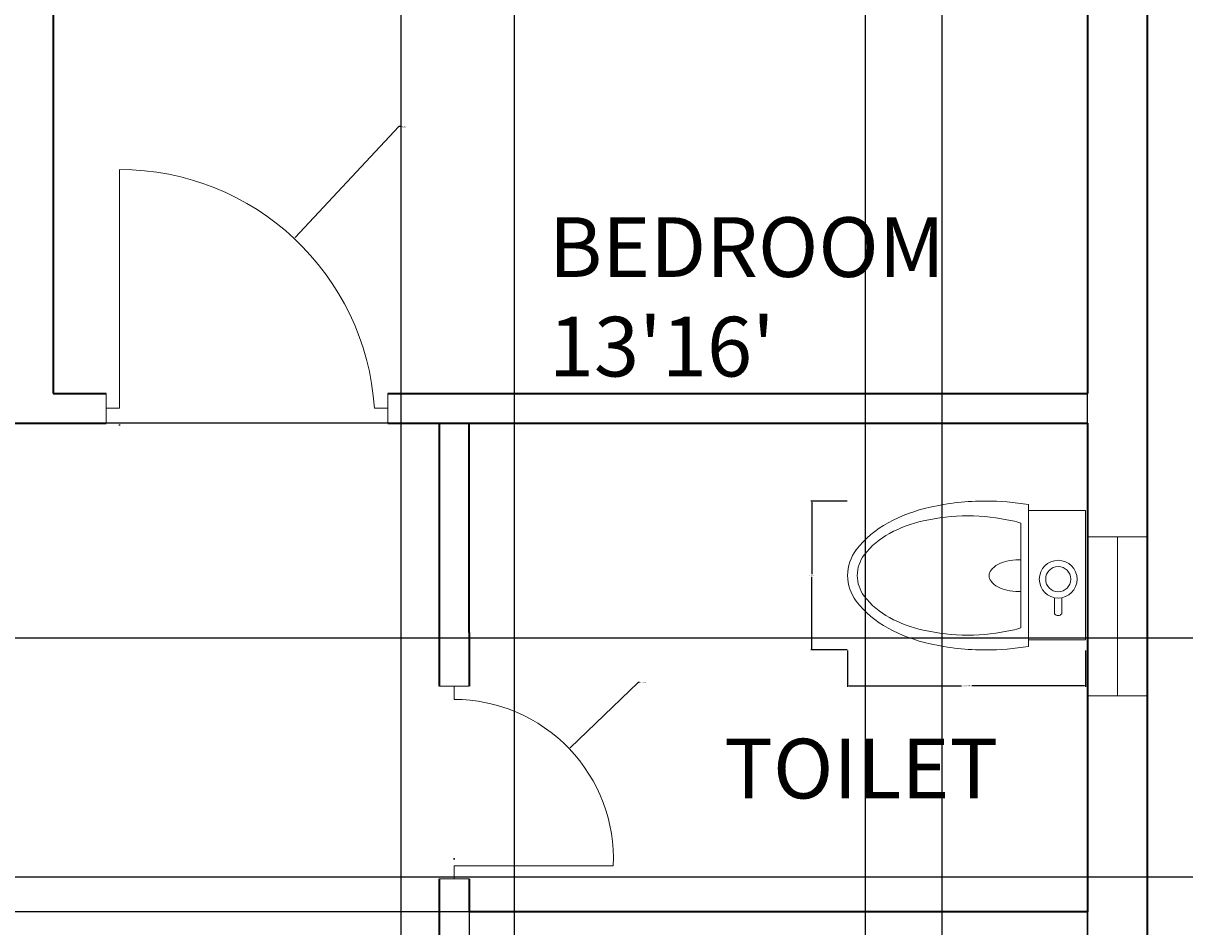
# Model space of a CAD drawing. Units: inches. Extents: x 1770 to 2988, y 1161 to 3221.
# Tile 22 of 44: x 2456 to 2631, y 2095 to 2231. Entities that reach past the tile are written whole.
import ezdxf

# ---------------------------------------------------------------- set-up
doc = ezdxf.new("R2010")
doc.units = ezdxf.units.IN
for name, color, linetype, lineweight in [('A-ANNO-DIMS', 2, 'Continuous', 18), ('A-AREA-IDEN', 7, 'Continuous', 18), ('A-DOOR', 4, 'Continuous', 18), ('A-FLOR-FIXT', 9, 'Continuous', 18), ('A-GLAZ', 4, 'Continuous', 18), ('A-WALL', 7, 'Continuous', 35)]:
    doc.layers.add(name, color=color, linetype=linetype, lineweight=lineweight)
doc.styles.get("Standard").update_dxf_attribs({"font": 'arial.ttf'})
doc.dimstyles.get("Standard").update_dxf_attribs({"dimtxt": 0.18, "dimasz": 0.18, "dimexe": 0.18, "dimexo": 0.0625, "dimgap": 0.09, "dimtad": 0, "dimtih": 1, "dimtoh": 1, "dimdec": 4, "dimzin": 0, "dimdsep": 46, "dimtxsty": 'Standard', "dimcen": 0.09, "dimadec": 0, "dimazin": 0, "dimtfac": 1, "dimtdec": 4, "dimtofl": 0, "dimtmove": 0, "dimatfit": 3, "dimfxl": 1, "dimtolj": 1, "dimtzin": 0, "dimarcsym": 0})

# ---------------------------------------------------------------- blocks, each defined once
blk = doc.blocks.new('A$C7FD35E1A')
for p, q in [((0.0233, 0.5799), (0.0233, 0.4408)), ((0.0233, 0.5799), (0.338, 0.5799)), ((0.338, 0.5799), (0.338, 0.4408)), ((0.2357, 0.5217), (0.2745, 0.5217)), ((0.2356, 0.5044), (0.275, 0.5044)), ((0.3542, 0.4408), (0.0087, 0.4408)), ((0.3093, 0.4224), (0.0536, 0.4224))]:
    blk.add_line(p, q)
for radius in [0.046, 0.0305]:
    blk.add_circle((0.1904, 0.5132), radius)
for centre, radius, start, end in [((0.2685, 0.5129), 0.0107, 307.488, 55.394), ((0.6238, 0.337), 0.6238, 170.4184, 180), ((-0.261, 0.337), 0.6238, 0, 9.5816), ((0.5354, 0.2931), 0.4991, 167.4267, 180), ((0.3603, 0.3321), 0.3197, 163.5954, 167.4267), ((0.277, 0.4171), 0.1337, 177.7133, 180), ((0.277, 0.4171), 0.1337, 180, 192.5399), ((0.0869, 0.4171), 0.1337, 347.4601, 0), ((0.0869, 0.4171), 0.1337, 360, 2.2867), ((0.0026, 0.3321), 0.3197, 12.5733, 16.4046), ((-0.1725, 0.2931), 0.4991, 0, 12.5733), ((0.23, 0.4066), 0.0855, 192.5399, 208.2349), ((0.1339, 0.4066), 0.0855, 331.7651, 347.4601), ((0.2004, 0.3907), 0.052, 208.2349, 232.3543), ((0.182, 0.3668), 0.0218, 232.3543, 270), ((0.182, 0.3668), 0.0218, 270, 307.6457), ((0.1635, 0.3907), 0.052, 307.6457, 331.7651), ((0.6238, 0.337), 0.6238, 180, 192.5733), ((-0.261, 0.337), 0.6238, 347.4267, 0), ((0.5354, 0.2931), 0.4991, 180, 192.5733), ((-0.1725, 0.2931), 0.4991, 347.4267, 0), ((0.405, 0.2881), 0.3996, 192.5733, 208.3008), ((-0.0421, 0.2881), 0.3996, 331.6992, 347.4267), ((0.3603, 0.254), 0.3197, 192.5733, 208.3008), ((0.0026, 0.254), 0.3197, 331.6992, 347.4267), ((0.2672, 0.214), 0.2432, 208.3008, 232.4306), ((0.2501, 0.1947), 0.1945, 208.3008, 232.4306), ((0.1128, 0.1947), 0.1945, 307.5694, 331.6992), ((0.0957, 0.214), 0.2432, 307.5694, 331.6992), ((0.1814, 0.1055), 0.082, 232.4306, 270), ((0.1814, 0.1055), 0.082, 270, 307.5694), ((0.1814, 0.1024), 0.1024, 232.4306, 270), ((0.1814, 0.1024), 0.1024, 270, 307.5694)]:
    blk.add_arc(centre, radius, start, end)
blk = doc.blocks.new('WIN-24-EXT')
for p, q in [((0, 9), (0, 0)), ((24, 4.5), (24, 9)), ((24, 9), (24, 0)), ((0, 0), (0, 4.5)), ((0, 4.5), (24, 4.5))]:
    blk.add_line(p, q)
blk = doc.blocks.new('*D40')
at = {"layer": 'A-ANNO-DIMS', "color": 0, "lineweight": -2, "transparency": 16777216}
for p, q in [((2580.5, 2136.95), (2580.5, 2131.45)), ((2616.39, 2136.95), (2616.39, 2131.45)), ((2580.68, 2131.63), (2597.67, 2131.63)), ((2616.21, 2131.63), (2599.22, 2131.63))]:
    blk.add_line(p, q, dxfattribs=at)
at = {"layer": 'A-ANNO-DIMS', "color": 0, "transparency": 16777216}
for points in [[(2580.68, 2131.66), (2580.68, 2131.6), (2580.5, 2131.63)], [(2616.21, 2131.66), (2616.21, 2131.6), (2616.39, 2131.63)]]:
    blk.add_solid(points, dxfattribs=at)
at = {"layer": 'Defpoints', "color": 0, "transparency": 16777216}
for p in [(2580.5, 2137.02), (2616.39, 2137.02), (2616.39, 2131.63)]:
    blk.add_point(p, dxfattribs=at)
at = {"layer": 'A-ANNO-DIMS', "color": 0, "transparency": 16777216, "insert": (2598.45, 2131.63), "char_height": 0.18, "attachment_point": 5}
blk.add_mtext('\\A1;WC 36 TYP.', dxfattribs=at)
blk = doc.blocks.new('*D41')
at = {"layer": 'A-ANNO-DIMS', "color": 0, "lineweight": -2, "transparency": 16777216}
for p, q in [((2580.44, 2159.47), (2574.94, 2159.47)), ((2575.12, 2159.29), (2575.12, 2148.43)), ((2575.12, 2137.2), (2575.12, 2148.07)), ((2580.44, 2137.02), (2574.94, 2137.02))]:
    blk.add_line(p, q, dxfattribs=at)
at = {"layer": 'A-ANNO-DIMS', "color": 0, "transparency": 16777216}
for points in [[(2575.09, 2159.29), (2575.15, 2159.29), (2575.12, 2159.47)], [(2575.09, 2137.2), (2575.15, 2137.2), (2575.12, 2137.02)]]:
    blk.add_solid(points, dxfattribs=at)
at = {"layer": 'Defpoints', "color": 0, "transparency": 16777216}
for p in [(2580.5, 2159.47), (2575.12, 2137.02), (2580.5, 2137.02)]:
    blk.add_point(p, dxfattribs=at)
at = {"layer": 'A-ANNO-DIMS', "color": 0, "transparency": 16777216, "insert": (2575.12, 2148.25), "char_height": 0.18, "attachment_point": 5}
blk.add_mtext('\\A1;22 TYP.', dxfattribs=at)
blk = doc.blocks.new('*D61')
at = {"layer": 'A-ANNO-DIMS', "color": 0, "lineweight": -2, "transparency": 16777216}
for p, q in [((2625.76, 2376.7), (2866.87, 2376.7)), ((2866.69, 2376.52), (2866.69, 1993.63)), ((2866.69, 1610.38), (2866.69, 1993.27)), ((2625.76, 1610.2), (2866.87, 1610.2))]:
    blk.add_line(p, q, dxfattribs=at)
at = {"layer": 'A-ANNO-DIMS', "color": 0, "transparency": 16777216}
for points in [[(2866.66, 2376.52), (2866.72, 2376.52), (2866.69, 2376.7)], [(2866.66, 1610.38), (2866.72, 1610.38), (2866.69, 1610.2)]]:
    blk.add_solid(points, dxfattribs=at)
at = {"layer": 'Defpoints', "color": 0, "transparency": 16777216}
for p in [(2625.7, 2376.7), (2866.69, 2376.7), (2625.7, 1610.2)]:
    blk.add_point(p, dxfattribs=at)
at = {"layer": 'A-ANNO-DIMS', "color": 0, "transparency": 16777216, "insert": (2866.69, 1993.45), "char_height": 0.18, "attachment_point": 5}
blk.add_mtext('\\A1;766.5', dxfattribs=at)
blk = doc.blocks.new('*D74')
at = {"layer": 'A-ANNO-DIMS', "color": 0, "lineweight": -2, "transparency": 16777216}
for p, q in [((2523.42, 2097.48), (2523.42, 1165.57)), ((2616.7, 2097.48), (2616.7, 1165.57)), ((2523.6, 1165.75), (2569.66, 1165.75)), ((2616.52, 1165.75), (2570.45, 1165.75))]:
    blk.add_line(p, q, dxfattribs=at)
at = {"layer": 'A-ANNO-DIMS', "color": 0, "transparency": 16777216}
for points in [[(2523.6, 1165.78), (2523.6, 1165.72), (2523.42, 1165.75)], [(2616.52, 1165.78), (2616.52, 1165.72), (2616.7, 1165.75)]]:
    blk.add_solid(points, dxfattribs=at)
at = {"layer": 'Defpoints', "color": 0, "transparency": 16777216}
for p in [(2523.42, 2097.54), (2616.7, 2097.54), (2616.7, 1165.75)]:
    blk.add_point(p, dxfattribs=at)
at = {"layer": 'A-ANNO-DIMS', "color": 0, "transparency": 16777216, "insert": (2570.06, 1165.75), "char_height": 0.18, "attachment_point": 5}
blk.add_mtext('\\A1;93.28', dxfattribs=at)
blk = doc.blocks.new('*D75')
at = {"layer": 'A-ANNO-DIMS', "color": 0, "lineweight": -2, "transparency": 16777216}
for p, q in [((2523.36, 2171.2), (1907.1, 2171.2)), ((1907.28, 2171.02), (1907.28, 2134.56)), ((1907.28, 2097.72), (1907.28, 2134.19)), ((2523.36, 2097.54), (1907.1, 2097.54))]:
    blk.add_line(p, q, dxfattribs=at)
at = {"layer": 'A-ANNO-DIMS', "color": 0, "transparency": 16777216}
for points in [[(1907.25, 2171.02), (1907.31, 2171.02), (1907.28, 2171.2)], [(1907.25, 2097.72), (1907.31, 2097.72), (1907.28, 2097.54)]]:
    blk.add_solid(points, dxfattribs=at)
at = {"layer": 'Defpoints', "color": 0, "transparency": 16777216}
for p in [(2523.42, 2171.2), (1907.28, 2097.54), (2523.42, 2097.54)]:
    blk.add_point(p, dxfattribs=at)
at = {"layer": 'A-ANNO-DIMS', "color": 0, "transparency": 16777216, "insert": (1907.28, 2134.37), "char_height": 0.18, "attachment_point": 5}
blk.add_mtext('\\A1;73.66', dxfattribs=at)
blk = doc.blocks.new('*D82')
at = {"layer": 'A-ANNO-DIMS', "color": 0, "lineweight": -2, "transparency": 16777216}
for p, q in [((2443.39, 1610.26), (2443.39, 2570.7)), ((2443.57, 2570.52), (2486.45, 2570.52)), ((2530.12, 2570.52), (2487.24, 2570.52)), ((2530.3, 1610.26), (2530.3, 2570.7))]:
    blk.add_line(p, q, dxfattribs=at)
at = {"layer": 'A-ANNO-DIMS', "color": 0, "transparency": 16777216}
for points in [[(2443.57, 2570.55), (2443.57, 2570.49), (2443.39, 2570.52)], [(2530.12, 2570.55), (2530.12, 2570.49), (2530.3, 2570.52)]]:
    blk.add_solid(points, dxfattribs=at)
at = {"layer": 'Defpoints', "color": 0, "transparency": 16777216}
for p in [(2530.3, 2570.52), (2443.39, 1610.2), (2530.3, 1610.2)]:
    blk.add_point(p, dxfattribs=at)
at = {"layer": 'A-ANNO-DIMS', "color": 0, "transparency": 16777216, "insert": (2486.85, 2570.52), "char_height": 0.18, "attachment_point": 5}
blk.add_mtext('\\A1;86.92', dxfattribs=at)
blk = doc.blocks.new('*D84')
at = {"layer": 'A-ANNO-DIMS', "color": 0, "lineweight": -2, "transparency": 16777216}
for p, q in [((2513.2, 1835.26), (2513.2, 2570.7)), ((2513.38, 2570.52), (2564.56, 2570.52)), ((2616.52, 2570.52), (2565.33, 2570.52)), ((2616.7, 1835.26), (2616.7, 2570.7))]:
    blk.add_line(p, q, dxfattribs=at)
at = {"layer": 'A-ANNO-DIMS', "color": 0, "transparency": 16777216}
for points in [[(2513.38, 2570.55), (2513.38, 2570.49), (2513.2, 2570.52)], [(2616.52, 2570.55), (2616.52, 2570.49), (2616.7, 2570.52)]]:
    blk.add_solid(points, dxfattribs=at)
at = {"layer": 'Defpoints', "color": 0, "transparency": 16777216}
for p in [(2616.7, 2570.52), (2513.2, 1835.2), (2616.7, 1835.2)]:
    blk.add_point(p, dxfattribs=at)
at = {"layer": 'A-ANNO-DIMS', "color": 0, "transparency": 16777216, "insert": (2564.95, 2570.52), "char_height": 0.18, "attachment_point": 5}
blk.add_mtext('\\A1;103.5', dxfattribs=at)
blk = doc.blocks.new('*D86')
at = {"layer": 'A-ANNO-DIMS', "color": 0, "lineweight": -2, "transparency": 16777216}
for p, q in [((2583.2, 1775.21), (2583.2, 2570.7)), ((2583.38, 2570.52), (2599.62, 2570.52)), ((2616.52, 2570.52), (2600.27, 2570.52)), ((2616.7, 1775.26), (2616.7, 2570.7))]:
    blk.add_line(p, q, dxfattribs=at)
at = {"layer": 'A-ANNO-DIMS', "color": 0, "transparency": 16777216}
for points in [[(2583.38, 2570.55), (2583.38, 2570.49), (2583.2, 2570.52)], [(2616.52, 2570.55), (2616.52, 2570.49), (2616.7, 2570.52)]]:
    blk.add_solid(points, dxfattribs=at)
at = {"layer": 'Defpoints', "color": 0, "transparency": 16777216}
for p in [(2616.7, 2570.52), (2583.2, 1775.15), (2616.7, 1775.2)]:
    blk.add_point(p, dxfattribs=at)
at = {"layer": 'A-ANNO-DIMS', "color": 0, "transparency": 16777216, "insert": (2599.95, 2570.52), "char_height": 0.18, "attachment_point": 5}
blk.add_mtext('\\A1;33.5', dxfattribs=at)
blk = doc.blocks.new('*D87')
at = {"layer": 'A-ANNO-DIMS', "color": 0, "lineweight": -2, "transparency": 16777216}
for p, q in [((2594.75, 1861.4), (2594.75, 2570.7)), ((2594.93, 2570.52), (2605.33, 2570.52)), ((2616.52, 2570.52), (2606.12, 2570.52)), ((2616.7, 1839.76), (2616.7, 2570.7))]:
    blk.add_line(p, q, dxfattribs=at)
at = {"layer": 'A-ANNO-DIMS', "color": 0, "transparency": 16777216}
for points in [[(2594.93, 2570.55), (2594.93, 2570.49), (2594.75, 2570.52)], [(2616.52, 2570.55), (2616.52, 2570.49), (2616.7, 2570.52)]]:
    blk.add_solid(points, dxfattribs=at)
at = {"layer": 'Defpoints', "color": 0, "transparency": 16777216}
for p in [(2616.7, 2570.52), (2594.75, 1861.34), (2616.7, 1839.7)]:
    blk.add_point(p, dxfattribs=at)
at = {"layer": 'A-ANNO-DIMS', "color": 0, "transparency": 16777216, "insert": (2605.72, 2570.52), "char_height": 0.18, "attachment_point": 5}
blk.add_mtext('\\A1;21.95', dxfattribs=at)
blk = doc.blocks.new('*D89')
at = {"layer": 'A-ANNO-DIMS', "color": 0, "lineweight": -2, "transparency": 16777216}
for p, q in [((2160.76, 2138.84), (2866.87, 2138.84)), ((2866.69, 2138.66), (2866.69, 2121.02)), ((2866.69, 2103.02), (2866.69, 2120.66)), ((2160.76, 2102.84), (2866.87, 2102.84))]:
    blk.add_line(p, q, dxfattribs=at)
at = {"layer": 'A-ANNO-DIMS', "color": 0, "transparency": 16777216}
for points in [[(2866.66, 2138.66), (2866.72, 2138.66), (2866.69, 2138.84)], [(2866.66, 2103.02), (2866.72, 2103.02), (2866.69, 2102.84)]]:
    blk.add_solid(points, dxfattribs=at)
at = {"layer": 'Defpoints', "color": 0, "transparency": 16777216}
for p in [(2160.7, 2138.84), (2866.69, 2138.84), (2160.7, 2102.84)]:
    blk.add_point(p, dxfattribs=at)
at = {"layer": 'A-ANNO-DIMS', "color": 0, "transparency": 16777216, "insert": (2866.69, 2120.84), "char_height": 0.18, "attachment_point": 5}
blk.add_mtext('\\A1;36', dxfattribs=at)
blk = doc.blocks.new('*D111')
at = {"layer": 'A-ANNO-DIMS', "color": 0, "lineweight": -2, "transparency": 16777216}
for p, q in [((2512.85, 2215.91), (2497.18, 2199.18)), ((2513.03, 2215.91), (2512.85, 2215.91)), ((2470.64, 2170.94), (2470.82, 2170.94)), ((2470.73, 2170.85), (2470.73, 2171.03))]:
    blk.add_line(p, q, dxfattribs=at)
at = {"layer": 'A-ANNO-DIMS', "color": 0, "transparency": 16777216}
blk.add_solid([(2497.16, 2199.2), (2497.2, 2199.16), (2497.06, 2199.05)], dxfattribs=at)
at = {"layer": 'Defpoints', "color": 0, "transparency": 16777216}
for p in [(2497.06, 2199.05), (2470.73, 2170.94)]:
    blk.add_point(p, dxfattribs=at)
at = {"layer": 'A-ANNO-DIMS', "color": 0, "transparency": 16777216, "insert": (2513.5, 2215.91), "char_height": 0.18, "attachment_point": 5}
blk.add_mtext('\\A1;R38.51', dxfattribs=at)
blk = doc.blocks.new('*D114')
at = {"layer": 'A-ANNO-DIMS', "color": 0, "lineweight": -2, "transparency": 16777216}
for p, q in [((2548.93, 2132.12), (2538.65, 2122.28)), ((2549.11, 2132.12), (2548.93, 2132.12)), ((2521.08, 2105.54), (2521.26, 2105.54)), ((2521.17, 2105.45), (2521.17, 2105.63))]:
    blk.add_line(p, q, dxfattribs=at)
at = {"layer": 'A-ANNO-DIMS', "color": 0, "transparency": 16777216}
blk.add_solid([(2538.63, 2122.3), (2538.67, 2122.26), (2538.52, 2122.15)], dxfattribs=at)
at = {"layer": 'Defpoints', "color": 0, "transparency": 16777216}
for p in [(2538.52, 2122.15), (2521.17, 2105.54)]:
    blk.add_point(p, dxfattribs=at)
at = {"layer": 'A-ANNO-DIMS', "color": 0, "transparency": 16777216, "insert": (2549.66, 2132.12), "char_height": 0.18, "attachment_point": 5}
blk.add_mtext('\\A1;R24.023', dxfattribs=at)

msp = doc.modelspace()

# ---------------------------------------------------------------- linework, layer by layer
at = {"layer": 'A-DOOR'}
for p, q in [((2470.7272, 2173.4521), (2470.7272, 2209.4521)), ((2468.7272, 2175.7021), (2468.7272, 2171.2021)), ((2511.1573, 2175.7021), (2511.1573, 2171.2021)), ((2468.7272, 2173.4521), (2470.7272, 2173.4521)), ((2511.1573, 2173.4521), (2509.1573, 2173.4521)), ((2511.1573, 2171.2021), (2511.1573, 2173.4521)), ((2518.9179, 2131.5604), (2523.4179, 2131.5604)), ((2523.4179, 2131.5604), (2521.1679, 2131.5604)), ((2521.1679, 2131.5604), (2521.1679, 2129.5604)), ((2521.1679, 2102.4974), (2521.1679, 2104.4974)), ((2521.1679, 2104.4974), (2545.1679, 2104.4974)), ((2523.4179, 2102.4974), (2518.9179, 2102.4974)), ((2518.9179, 2102.4974), (2521.1679, 2102.4974))]:
    msp.add_line(p, q, dxfattribs=at)
for centre, radius, start in [((2470.7272, 2170.9399), 38.5122, 3.740137), ((2521.1679, 2105.5378), 24.0225, 357.517781)]:
    msp.add_arc(centre, radius, start, 90, dxfattribs=at)
at = {"layer": 'A-WALL'}
for p, q in [((2625.696, 2376.7021), (2625.696, 1610.2021)), ((2460.696, 2367.7021), (2460.696, 2175.7021)), ((2616.696, 2367.7021), (2616.696, 2175.7021)), ((2460.696, 2175.7021), (2468.7272, 2175.7021)), ((2511.1573, 2175.7021), (2616.696, 2175.7021)), ((2323.4422, 2171.2021), (2468.7272, 2171.2021)), ((2511.1573, 2171.2021), (2616.696, 2171.2021)), ((2518.9179, 2171.2021), (2518.9179, 2139.6736)), ((2523.4179, 2139.6736), (2523.4179, 2171.2021)), ((2616.696, 2171.2021), (2616.696, 2097.5443)), ((2518.9179, 2139.6736), (2518.9179, 2131.5604)), ((2523.4179, 2139.6736), (2523.4179, 2131.5604)), ((2518.9179, 2102.4974), (2518.9179, 2097.5443)), ((2523.4179, 2102.4974), (2523.4179, 2097.5443)), ((2518.9179, 2097.5443), (2518.9179, 2070.4236)), ((2616.696, 2097.5443), (2523.4179, 2097.5443))]:
    msp.add_line(p, q, dxfattribs=at)

# ---------------------------------------------------------------- block references
at = {"layer": 'A-FLOR-FIXT', "xscale": 61.88350044382122, "yscale": 61.88350044382122, "zscale": 61.88350044382122, "rotation": 270}
msp.add_blockref('A$C7FD35E1A', (2580.5028, 2159.4737), dxfattribs=at)
at = {"layer": 'A-GLAZ', "rotation": 270}
msp.add_blockref('WIN-24-EXT', (2616.6958, 2154.0926), dxfattribs=at)

# ---------------------------------------------------------------- texts
at = {"layer": 'A-AREA-IDEN', "char_height": 9, "attachment_point": 1}
for s, width, insert in [("BEDROOM\\P13'16'", 88.118515, (2535.4437, 2202.2494)), ('TOILET', 73.917952, (2561.9059, 2123.6371))]:
    msp.add_mtext_dynamic_manual_height_columns(s, width=width, gutter_width=12.5, heights=[0], dxfattribs=dict(at, insert=insert))

# ---------------------------------------------------------------- dimensions: what is measured, and where the dimension line sits
at = {"layer": 'A-ANNO-DIMS'}
for base, p1, p2, override, picture, middle in [((2530.3038, 2570.5247), (2443.3863, 1610.2021), (2530.3038, 1610.2021), {"dimdec": 2, "dimlfac": 1, "dimrnd": 0, "dimzin": 0, "dimdsep": 46, "dimlunit": 2}, '*D82', (2486.8451, 2570.5247)), ((2616.696, 2570.5247), (2513.196, 1835.2021), (2616.696, 1835.2021), {"dimdec": 1, "dimlfac": 1, "dimrnd": 0, "dimzin": 0, "dimdsep": 46, "dimlunit": 2}, '*D84', (2564.946, 2570.5247)), ((2616.696, 2570.5247), (2583.196, 1775.149), (2616.696, 1775.2021), {"dimdec": 1, "dimlfac": 1, "dimrnd": 0, "dimzin": 0, "dimdsep": 46, "dimlunit": 2}, '*D86', (2599.946, 2570.5247)), ((2616.696, 2570.5247), (2594.7479, 1861.3395), (2616.696, 1839.7021), {"dimdec": 2, "dimlfac": 1, "dimrnd": 0, "dimzin": 0, "dimdsep": 46, "dimlunit": 2}, '*D87', (2605.7219, 2570.5247)), ((2616.696, 1165.752), (2523.4179, 2097.5443), (2616.696, 2097.5443), {"dimdec": 2, "dimlfac": 1, "dimrnd": 0, "dimzin": 0, "dimdsep": 46, "dimlunit": 2}, '*D74', (2570.0569, 1165.752))]:
    dim = msp.add_linear_dim(base=base, p1=p1, p2=p2, dimstyle='Standard', override=override, dxfattribs=at)
    dim.commit()
    dim.dimension.update_dxf_attribs({"geometry": picture, "text_midpoint": middle})
for base, p1, p2, override, picture, middle in [((2866.6874, 2376.7021), (2625.696, 1610.2021), (2625.696, 2376.7021), {"dimdec": 1, "dimlfac": 1, "dimrnd": 0, "dimzin": 0, "dimdsep": 46, "dimlunit": 2}, '*D61', (2866.6874, 1993.4521)), ((1907.2844, 2097.5443), (2523.4179, 2171.2021), (2523.4179, 2097.5443), {"dimdec": 2, "dimlfac": 1, "dimrnd": 0, "dimzin": 0, "dimdsep": 46, "dimlunit": 2}, '*D75', (1907.2844, 2134.3732)), ((2866.6874, 2138.8392), (2160.696, 2102.8392), (2160.696, 2138.8392), {"dimdec": 0, "dimlfac": 1, "dimrnd": 0, "dimzin": 0, "dimdsep": 46, "dimlunit": 2}, '*D89', (2866.6874, 2120.8392))]:
    dim = msp.add_linear_dim(base=base, p1=p1, p2=p2, angle=90, dimstyle='Standard', override=override, dxfattribs=at)
    dim.commit()
    dim.dimension.update_dxf_attribs({"geometry": picture, "text_midpoint": middle})
for center, mpoint, override, picture, middle in [((2470.7272, 2170.9399), (2497.0563, 2199.0463), {"dimdec": 2, "dimlfac": 1, "dimrnd": 0, "dimzin": 0, "dimdsep": 46, "dimlunit": 2}, '*D111', (2513.4962, 2215.9101)), ((2521.1679, 2105.5378), (2538.5184, 2122.1524), {"dimdec": 3, "dimlfac": 1, "dimrnd": 0, "dimzin": 0, "dimdsep": 46, "dimlunit": 2}, '*D114', (2549.6585, 2132.1211))]:
    dim = msp.add_radius_dim(center=center, mpoint=mpoint, dimstyle='Standard', override=override, dxfattribs=at)
    dim.commit()
    dim.dimension.update_dxf_attribs({"geometry": picture, "text_midpoint": middle, "dimtype": 164})
dim = msp.add_linear_dim(base=(2575.1196, 2137.0174), p1=(2580.5028, 2159.4737), p2=(2580.5028, 2137.0174), angle=270, text='<> TYP.', dimstyle='Standard', override={"dimdec": 0, "dimlfac": 1, "dimrnd": 0, "dimzin": 0, "dimdsep": 46, "dimlunit": 2}, dxfattribs=at)
dim.commit()
dim.dimension.update_dxf_attribs({"geometry": '*D41', "text_midpoint": (2575.1196, 2148.2455)})
dim = msp.add_linear_dim(base=(2616.3909, 2131.6342), p1=(2580.5028, 2137.0174), p2=(2616.3909, 2137.0174), text='WC <> TYP.', dimstyle='Standard', override={"dimdec": 0, "dimlfac": 1, "dimrnd": 0, "dimzin": 0, "dimdsep": 46, "dimlunit": 2}, dxfattribs=at)
dim.commit()
dim.dimension.update_dxf_attribs({"geometry": '*D40', "text_midpoint": (2598.4469, 2131.6342)})

doc.saveas('drawing.dxf')
